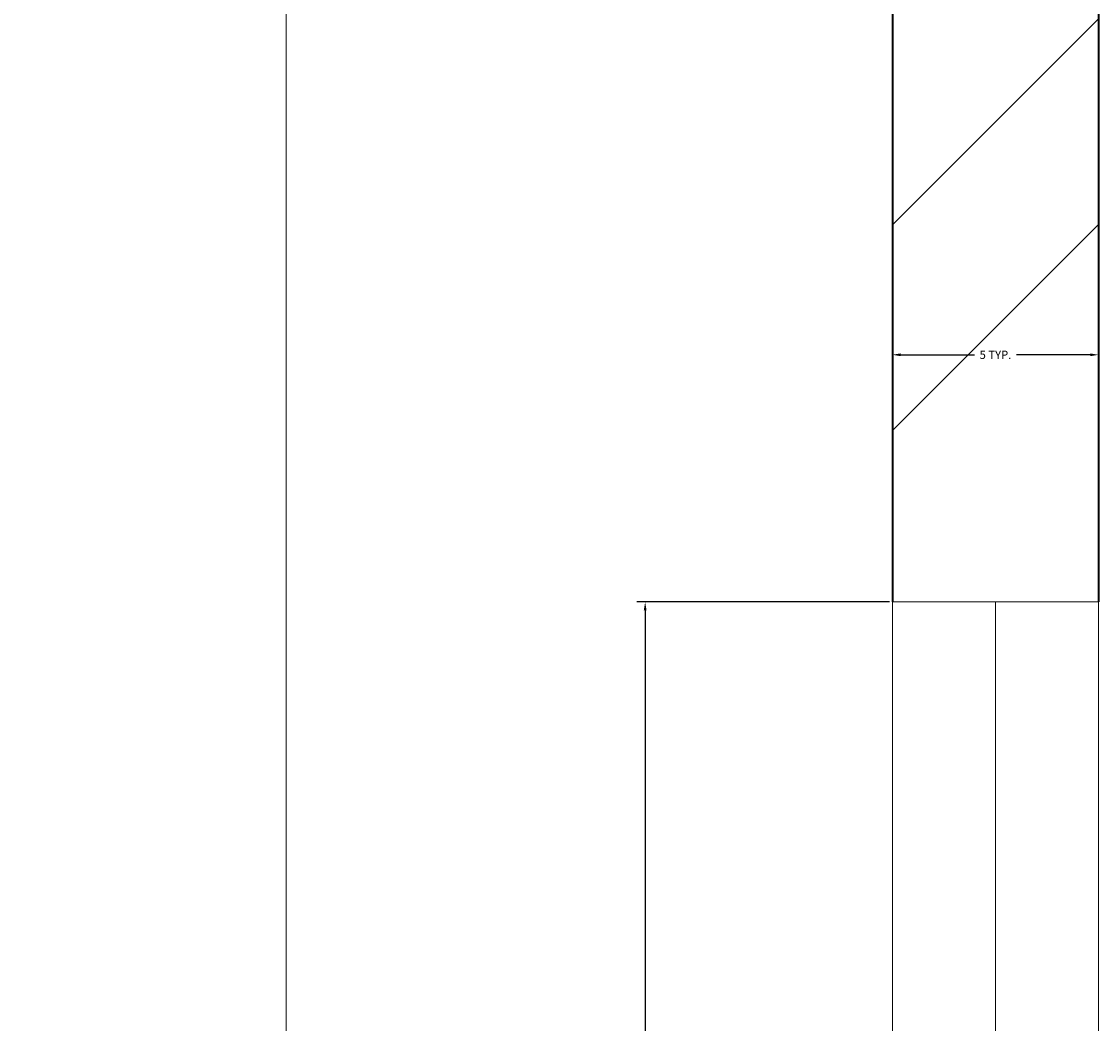
# Model space of a CAD drawing. Units: inches. Extents: x 1885 to 2748, y 783 to 2421.
# Tile 114 of 117: x 2595 to 2618, y 2071 to 2093. Entities that reach past the tile are written whole.
import ezdxf

# ---------------------------------------------------------------- set-up
doc = ezdxf.new("R2010")
doc.units = ezdxf.units.IN
for name, color, linetype, lineweight in [('A-ANNO-DIMS', 2, 'Continuous', 18), ('A-FLOR-CASE', 9, 'Continuous', 18), ('A-GLAZ', 181, 'Continuous', 18), ('A-WALL', 7, 'Continuous', 35)]:
    doc.layers.add(name, color=color, linetype=linetype, lineweight=lineweight)
doc.layers.add('A-WALL-PATT', color=85, linetype='Continuous', lineweight=13, true_color=0x58ba48)
doc.styles.get("Standard").update_dxf_attribs({"font": 'arial.ttf'})
doc.dimstyles.get("Standard").update_dxf_attribs({"dimtxt": 0.18, "dimasz": 0.18, "dimexe": 0.18, "dimexo": 0.0625, "dimgap": 0.09, "dimtad": 0, "dimtih": 1, "dimtoh": 1, "dimdec": 4, "dimzin": 0, "dimdsep": 46, "dimtxsty": 'Standard', "dimcen": 0.09, "dimadec": 0, "dimazin": 0, "dimtfac": 1, "dimtdec": 4, "dimtofl": 0, "dimtmove": 0, "dimatfit": 3, "dimfxl": 1, "dimtolj": 1, "dimtzin": 0, "dimarcsym": 0})

# ---------------------------------------------------------------- blocks, each defined once
blk = doc.blocks.new('WIN-36-ALT')
for p, q in [((0.004, 35.998), (4.504, 35.998)), ((0.004, 35.998), (0.004, -0.002)), ((4.504, 35.998), (2.254, 35.998)), ((2.254, 35.998), (2.254, -0.002)), ((4.504, -0.002), (4.504, 35.998)), ((4.504, -0.002), (0.004, -0.002)), ((2.254, -0.002), (4.504, -0.002))]:
    blk.add_line(p, q)
blk = doc.blocks.new('*D21')
at = {"layer": 'A-ANNO-DIMS', "color": 0, "lineweight": -2, "transparency": 16777216}
for p, q in [((2613.711, 2080.19), (2608.194, 2080.19)), ((2608.374, 2080.01), (2608.374, 2062.373)), ((2608.374, 2044.37), (2608.374, 2062.007)), ((2613.711, 2044.19), (2608.194, 2044.19))]:
    blk.add_line(p, q, dxfattribs=at)
at = {"layer": 'A-ANNO-DIMS', "color": 0, "transparency": 16777216}
for points in [[(2608.344, 2080.01), (2608.404, 2080.01), (2608.374, 2080.19)], [(2608.344, 2044.37), (2608.404, 2044.37), (2608.374, 2044.19)]]:
    blk.add_solid(points, dxfattribs=at)
at = {"layer": 'Defpoints', "color": 0, "transparency": 16777216}
for p in [(2608.374, 2080.19), (2613.774, 2080.19), (2613.774, 2044.19)]:
    blk.add_point(p, dxfattribs=at)
at = {"layer": 'A-ANNO-DIMS', "color": 0, "transparency": 16777216, "insert": (2608.374, 2062.19), "char_height": 0.18, "attachment_point": 5}
blk.add_mtext('\\A1;ALT. WINDOW 36 TYP.', dxfattribs=at)
blk = doc.blocks.new('*D22')
at = {"layer": 'A-ANNO-DIMS', "color": 0, "lineweight": -2, "transparency": 16777216}
for p, q in [((2613.774, 2080.252), (2613.774, 2085.77)), ((2618.274, 2080.252), (2618.274, 2085.77)), ((2613.954, 2085.59), (2615.565, 2085.59)), ((2618.094, 2085.59), (2616.482, 2085.59))]:
    blk.add_line(p, q, dxfattribs=at)
at = {"layer": 'A-ANNO-DIMS', "color": 0, "transparency": 16777216}
for points in [[(2613.954, 2085.62), (2613.954, 2085.56), (2613.774, 2085.59)], [(2618.094, 2085.62), (2618.094, 2085.56), (2618.274, 2085.59)]]:
    blk.add_solid(points, dxfattribs=at)
at = {"layer": 'Defpoints', "color": 0, "transparency": 16777216}
for p in [(2618.274, 2085.59), (2613.774, 2080.19), (2618.274, 2080.19)]:
    blk.add_point(p, dxfattribs=at)
at = {"layer": 'A-ANNO-DIMS', "color": 0, "transparency": 16777216, "insert": (2616.024, 2085.59), "char_height": 0.18, "attachment_point": 5}
blk.add_mtext('\\A1;5 TYP.', dxfattribs=at)

msp = doc.modelspace()

# ---------------------------------------------------------------- hatches: boundary and pattern name
at = {"layer": 'A-WALL-PATT'}
h = msp.add_hatch(dxfattribs=at)
h.set_pattern_fill('ANSI32', color=256)
h.paths.add_polyline_path([(2007.772, 2318.006), (1980.774, 2318.006), (1980.774, 2281.215), (1985.274, 2281.215), (1985.274, 2313.506), (2007.772, 2313.506), (2007.772, 2315.756)])
h.paths.add_polyline_path([(2094.324, 2318.006), (2067.772, 2318.006), (2067.772, 2313.506), (2094.324, 2313.506), (2094.324, 2315.756)])
h.paths.add_polyline_path([(2131.367, 2315.756), (2131.367, 2318.006), (2131.189, 2318.006), (2112.609, 2318.006), (2112.609, 2313.506), (2117.274, 2313.506), (2117.274, 2255.201), (2121.774, 2255.201), (2121.774, 2313.506), (2131.367, 2313.506)])
h.paths.add_polyline_path([(2190.512, 2318.006), (2155.367, 2318.006), (2155.367, 2313.506), (2169.774, 2313.506), (2169.774, 2229.506), (2121.774, 2229.506), (2121.774, 2233.451), (2119.524, 2233.451), (2117.274, 2233.451), (2117.274, 2201.101), (2121.774, 2201.101), (2121.774, 2225.006), (2169.774, 2225.006), (2169.774, 2165.006), (2306.274, 2165.006), (2306.274, 2066.006), (2310.774, 2066.006), (2344.274, 2066.006), (2486.274, 2066.006), (2486.274, 1886.006), (2483.02, 1886.006), (2483.02, 1881.506), (2486.274, 1881.506), (2486.274, 1880.678), (2490.774, 1880.678), (2490.774, 2070.506), (2344.274, 2070.506), (2310.774, 2070.506), (2310.774, 2165.006), (2310.774, 2173.636), (2308.524, 2173.636), (2306.274, 2173.636), (2306.274, 2169.506), (2174.274, 2169.506), (2174.274, 2313.506), (2190.512, 2313.506), (2190.512, 2315.756)])
h.paths.add_polyline_path([(1985.274, 2221.215), (1980.774, 2221.215), (1980.774, 2165.006), (1992.774, 2165.006), (1992.774, 2141.927), (1997.274, 2141.927), (1997.274, 2165.006), (2117.274, 2165.006), (2117.274, 2163.126), (2121.774, 2163.126), (2121.774, 2172.734), (2119.524, 2172.734), (2117.274, 2172.734), (2117.274, 2169.506), (1985.274, 2169.506)])
h.paths.add_polyline_path([(1997.274, 2105.927), (1992.774, 2105.927), (1992.774, 2070.506), (2016.774, 2070.506), (2016.774, 2059.123), (2019.024, 2059.123), (2021.274, 2059.123), (2021.274, 2070.506), (2117.274, 2070.506), (2117.274, 2022.506), (2114.423, 2022.506), (2114.423, 2018.006), (2123.627, 2018.006), (2123.627, 2020.256), (2123.627, 2022.506), (2121.774, 2022.506), (2121.774, 2142.587), (2119.524, 2142.587), (2117.274, 2142.587), (2117.274, 2075.006), (1997.274, 2075.006)])
h.paths.add_polyline_path([(2092.029, 2020.256), (2092.029, 2022.506), (2021.274, 2022.506), (2021.274, 2035.123), (2016.774, 2035.123), (2016.774, 2018.006), (2016.774, 1978.784), (2021.274, 1978.784), (2021.274, 2018.006), (2092.029, 2018.006)])
h.paths.add_polyline_path([(2260.938, 2022.506), (2153.105, 2022.506), (2153.105, 2020.256), (2153.105, 2018.006), (2155.274, 2018.006), (2155.274, 1886.006), (2107.629, 1886.006), (2107.629, 1881.506), (2182.911, 1881.506), (2182.911, 1883.756), (2182.911, 1886.006), (2159.774, 1886.006), (2159.774, 2018.006), (2260.938, 2018.006), (2260.938, 2020.256)])
h.paths.add_polyline_path([(2047.629, 1883.756), (2047.629, 1886.006), (2021.274, 1886.006), (2021.274, 1918.784), (2019.024, 1918.784), (2016.774, 1918.784), (2016.774, 1881.506), (2047.629, 1881.506)])
h.paths.add_polyline_path([(2306.361, 1883.756), (2306.361, 1886.006), (2296.274, 1886.006), (2296.274, 1982.006), (2316.535, 1982.006), (2316.535, 1984.256), (2316.535, 1986.506), (2296.274, 1986.506), (2296.274, 2022.506), (2289.276, 2022.506), (2289.276, 2018.006), (2291.774, 2018.006), (2291.774, 1886.006), (2242.911, 1886.006), (2242.911, 1881.506), (2306.361, 1881.506)], flags=17)
h.paths.add_polyline_path([(1985.274, 1843.006), (2021.6, 1843.006), (2021.534, 1845.441), (2021.477, 1847.506), (1980.774, 1847.506), (1980.774, 1809.446), (1985.274, 1809.446)])
h.paths.add_polyline_path([(2131.482, 1845.256), (2131.482, 1847.506), (2081.534, 1847.506), (2081.534, 1843.006), (2117.274, 1843.006), (2117.274, 1784.147), (2119.524, 1784.147), (2121.774, 1784.147), (2121.774, 1843.006), (2131.482, 1843.006)])
h.paths.add_polyline_path([(2203.886, 1847.506), (2155.482, 1847.506), (2155.482, 1843.006), (2169.774, 1843.006), (2169.774, 1759.006), (2121.774, 1759.006), (2121.774, 1761.457), (2117.274, 1761.457), (2117.274, 1730.429), (2121.774, 1730.429), (2121.774, 1754.506), (2177.421, 1754.506), (2177.421, 1756.756), (2177.421, 1759.006), (2174.274, 1759.006), (2174.274, 1843.006), (2203.886, 1843.006)])
h.paths.add_polyline_path([(2335.554, 1845.256), (2335.554, 1847.506), (2239.886, 1847.506), (2239.886, 1843.006), (2306.274, 1843.006), (2306.274, 1759.006), (2199.486, 1759.006), (2199.486, 1754.506), (2310.774, 1754.506), (2310.774, 1843.006), (2335.554, 1843.006)])
h.paths.add_polyline_path([(2348.774, 2022.506), (2344.274, 2022.506), (2344.274, 1986.506), (2341.681, 1986.506), (2341.681, 1982.006), (2344.274, 1982.006), (2344.274, 1886.006), (2330.361, 1886.006), (2330.361, 1881.506), (2361.627, 1881.506), (2361.627, 1883.756), (2361.627, 1886.006), (2348.774, 1886.006)], flags=17)
h.paths.add_polyline_path([(2283.251, 2315.756), (2283.251, 2318.006), (2238.512, 2318.006), (2238.512, 2313.506), (2283.251, 2313.506)], flags=17)
h.paths.add_polyline_path([(2363.274, 2348.006), (2388.677, 2348.006), (2388.677, 2350.256), (2388.677, 2352.506), (2358.774, 2352.506), (2358.774, 2348.006), (2358.774, 2318.006), (2344.481, 2318.006), (2344.481, 2313.506), (2358.774, 2313.506), (2358.774, 2229.506), (2310.774, 2229.506), (2310.774, 2231.952), (2306.274, 2231.952), (2306.274, 2205.611), (2310.774, 2205.611), (2310.774, 2225.006), (2358.774, 2225.006), (2358.774, 2211.506), (2452.329, 2211.506), (2452.329, 2213.756), (2452.329, 2216.006), (2363.274, 2216.006), (2363.274, 2318.006)])
h.paths.add_polyline_path([(2310.774, 2313.506), (2320.481, 2313.506), (2320.481, 2315.756), (2320.481, 2318.006), (2302.728, 2318.006), (2302.728, 2313.506), (2306.274, 2313.506), (2306.274, 2251.076), (2310.774, 2251.076)], flags=17)
h.paths.add_polyline_path([(2490.774, 2352.506), (2486.274, 2352.506), (2448.677, 2352.506), (2448.677, 2348.006), (2486.274, 2348.006), (2486.274, 2318.006), (2486.274, 2216.006), (2481.78, 2216.006), (2481.78, 2211.506), (2486.274, 2211.506), (2486.274, 2165.006), (2493.289, 2165.006), (2493.289, 2167.256), (2493.289, 2169.506), (2490.774, 2169.506), (2490.774, 2313.506), (2494.429, 2313.506), (2494.429, 2318.006), (2490.774, 2318.006)])
h.paths.add_polyline_path([(2534.653, 2318.006), (2515.691, 2318.006), (2515.691, 2313.506), (2534.653, 2313.506), (2534.653, 2315.756)])
h.paths.add_polyline_path([(2618.274, 2318.006), (2594.653, 2318.006), (2594.653, 2313.506), (2613.774, 2313.506), (2613.774, 2281.706), (2618.274, 2281.706)])
h.paths.add_polyline_path([(2618.274, 2221.706), (2613.774, 2221.706), (2613.774, 2169.506), (2554.019, 2169.506), (2554.019, 2165.006), (2613.774, 2165.006), (2613.774, 2152.878), (2618.274, 2152.878)])
h.paths.add_polyline_path([(2618.274, 2128.878), (2616.024, 2128.878), (2613.774, 2128.878), (2613.774, 2117.006), (2529.774, 2117.006), (2529.774, 2165.006), (2532.848, 2165.006), (2532.848, 2169.506), (2522.867, 2169.506), (2522.867, 2165.006), (2525.274, 2165.006), (2525.274, 2117.006), (2525.274, 2112.506), (2525.274, 2108.576), (2529.774, 2108.576), (2529.774, 2112.506), (2613.774, 2112.506), (2613.774, 2080.19), (2618.274, 2080.19)])
h.paths.add_polyline_path([(2618.274, 2044.19), (2616.024, 2044.19), (2613.774, 2044.19), (2613.774, 2015.506), (2529.774, 2015.506), (2529.774, 2088.582), (2527.524, 2088.582), (2525.274, 2088.582), (2525.274, 2011.006), (2613.774, 2011.006), (2613.774, 1956.755), (2618.274, 1956.755)])
h.paths.add_polyline_path([(2618.274, 1881.506), (2618.274, 1896.755), (2613.774, 1896.755), (2613.774, 1881.506), (2613.774, 1847.506), (2592.715, 1847.506), (2592.715, 1843.006), (2613.774, 1843.006), (2613.774, 1765.006), (2613.774, 1760.506), (2609.621, 1760.506), (2609.621, 1756.006), (2613.774, 1756.006), (2613.774, 1660.006), (2608.544, 1660.006), (2608.544, 1655.506), (2613.774, 1655.506), (2613.774, 1508.158), (2618.274, 1508.158)])
h.paths.add_polyline_path([(2565.774, 1843.006), (2568.997, 1843.006), (2568.997, 1847.506), (2490.774, 1847.506), (2490.774, 1849.7), (2488.524, 1849.7), (2486.274, 1849.7), (2486.274, 1847.506), (2477.274, 1847.506), (2477.274, 1838.506), (2477.274, 1821.493), (2486.274, 1821.493), (2486.274, 1838.506), (2561.274, 1838.506), (2561.274, 1765.006), (2486.274, 1765.006), (2486.274, 1786.157), (2477.274, 1786.157), (2477.274, 1765.006), (2477.274, 1756.006), (2486.274, 1756.006), (2565.774, 1756.006), (2585.621, 1756.006), (2585.621, 1758.256), (2585.621, 1760.506), (2565.774, 1760.506), (2565.774, 1765.006)])
h.paths.add_polyline_path([(2486.274, 1651.006), (2561.274, 1651.006), (2561.274, 1567.006), (2486.274, 1567.006), (2486.274, 1591.321), (2477.274, 1591.321), (2477.274, 1567.006), (2477.274, 1558.006), (2477.274, 1555.439), (2481.774, 1555.439), (2481.774, 1558.006), (2568.653, 1558.006), (2568.653, 1560.256), (2568.653, 1562.506), (2565.774, 1562.506), (2565.774, 1655.506), (2584.544, 1655.506), (2584.544, 1657.756), (2584.544, 1660.006), (2565.774, 1660.006), (2486.274, 1660.006), (2477.274, 1660.006), (2477.274, 1651.006), (2477.274, 1632.989), (2486.274, 1632.989)])
h.paths.add_polyline_path([(2449.967, 1883.756), (2449.967, 1886.006), (2421.627, 1886.006), (2421.627, 1881.506), (2449.967, 1881.506)], flags=17)
h.paths.add_polyline_path([(2447.274, 1847.506), (2395.554, 1847.506), (2395.554, 1843.006), (2442.774, 1843.006), (2442.774, 1809.27), (2447.274, 1809.27)])
h.paths.add_polyline_path([(1985.274, 1749.446), (1980.774, 1749.446), (1980.774, 1694.504), (1985.274, 1694.504), (1985.274, 1694.506), (1986.897, 1694.506), (1986.897, 1697.78), (1986.897, 1699.006), (1985.274, 1699.006)])
h.paths.add_polyline_path([(2152.774, 1699.006), (2121.774, 1699.006), (2121.774, 1703.668), (2119.524, 1703.668), (2117.274, 1703.668), (2117.274, 1699.006), (2009.219, 1699.006), (2009.219, 1694.506), (2148.274, 1694.506), (2148.274, 1692.631), (2152.774, 1692.631)])
h.paths.add_polyline_path([(2016.274, 1694.506), (2011.774, 1694.506), (2011.774, 1558.006), (2040.806, 1558.006), (2040.806, 1560.256), (2040.806, 1562.506), (2016.274, 1562.506)])
h.paths.add_polyline_path([(2152.774, 1663.017), (2150.524, 1663.017), (2148.274, 1663.017), (2148.274, 1562.506), (2100.806, 1562.506), (2100.806, 1558.006), (2165.119, 1558.006), (2165.119, 1560.256), (2165.119, 1562.506), (2152.774, 1562.506), (2152.774, 1610.506), (2224.774, 1610.506), (2224.774, 1607.99), (2229.274, 1607.99), (2229.274, 1615.006), (2152.774, 1615.006)])
h.paths.add_polyline_path([(2238.613, 1560.256), (2238.613, 1562.506), (2229.274, 1562.506), (2229.274, 1588.756), (2227.024, 1588.763), (2224.774, 1588.771), (2224.774, 1562.506), (2189.119, 1562.506), (2189.119, 1558.006), (2238.613, 1558.006)])
h.paths.add_polyline_path([(2336.024, 1560.256), (2336.024, 1562.506), (2310.774, 1562.506), (2310.774, 1656.347), (2308.524, 1656.347), (2306.274, 1656.347), (2306.274, 1562.506), (2286.613, 1562.506), (2286.613, 1558.006), (2336.024, 1558.006)])
h.paths.add_polyline_path([(2447.274, 1690.968), (2445.024, 1690.968), (2442.774, 1690.968), (2442.774, 1687.006), (2306.274, 1687.006), (2306.274, 1680.75), (2310.774, 1680.75), (2310.774, 1682.506), (2442.774, 1682.506), (2442.774, 1562.506), (2396.024, 1562.506), (2396.024, 1558.006), (2447.274, 1558.006)])
h.paths.add_polyline_path([(2447.274, 1749.27), (2445.024, 1749.27), (2442.774, 1749.27), (2442.774, 1717.232), (2447.274, 1717.232)])
h.paths.add_polyline_path([(2044.674, 1521.756), (2044.674, 1524.006), (2007.274, 1524.006), (2007.274, 1503.49), (2009.524, 1503.49), (2011.774, 1503.49), (2011.774, 1519.506), (2044.674, 1519.506)])
h.paths.add_polyline_path([(2177.969, 1521.756), (2177.969, 1524.006), (2104.674, 1524.006), (2104.674, 1519.506), (2145.774, 1519.506), (2145.774, 1387.506), (2143.37, 1387.506), (2143.37, 1383.006), (2251.585, 1383.006), (2251.585, 1385.256), (2251.585, 1387.506), (2150.274, 1387.506), (2150.274, 1519.506), (2177.969, 1519.506)])
h.paths.add_polyline_path([(2298.704, 1524.006), (2237.969, 1524.006), (2237.969, 1519.506), (2282.274, 1519.506), (2282.274, 1387.506), (2279.683, 1387.506), (2279.683, 1383.006), (2286.774, 1383.006), (2286.774, 1419.006), (2312.451, 1419.006), (2312.451, 1421.256), (2312.451, 1423.506), (2286.774, 1423.506), (2286.774, 1519.506), (2298.704, 1519.506), (2298.704, 1521.722)], flags=17)
h.paths.add_polyline_path([(2361.897, 1521.756), (2361.897, 1524.006), (2322.704, 1524.006), (2322.704, 1519.506), (2334.774, 1519.506), (2334.774, 1423.506), (2331.93, 1423.506), (2331.93, 1419.006), (2334.774, 1419.006), (2334.774, 1387.506), (2334.774, 1383.228), (2339.274, 1383.228), (2339.274, 1387.506), (2339.274, 1519.506), (2361.897, 1519.506)], flags=17)
h.paths.add_polyline_path([(2447.274, 1521.756), (2447.274, 1524.006), (2421.897, 1524.006), (2421.897, 1519.506), (2447.274, 1519.506)], flags=17)
h.paths.add_polyline_path([(2481.774, 1529.6), (2479.524, 1529.6), (2477.274, 1529.6), (2477.274, 1524.006), (2474.489, 1524.006), (2474.489, 1519.506), (2477.274, 1519.506), (2477.274, 1334.506), (2296.774, 1334.506), (2296.774, 1240.506), (2160.274, 1240.506), (2160.274, 1180.506), (2112.274, 1180.506), (2112.274, 1207.692), (2110.024, 1207.692), (2107.774, 1207.692), (2107.774, 1171.609), (2112.274, 1171.609), (2112.274, 1176.006), (2160.274, 1176.006), (2160.274, 1092.006), (2144.221, 1092.006), (2144.221, 1087.506), (2189.497, 1087.506), (2189.497, 1089.756), (2189.497, 1092.006), (2164.774, 1092.006), (2164.774, 1236.006), (2296.774, 1236.006), (2296.774, 1231.912), (2301.274, 1231.912), (2301.274, 1330.006), (2481.774, 1330.006), (2481.774, 1387.506)])
h.paths.add_polyline_path([(2618.274, 1448.158), (2613.774, 1448.158), (2613.774, 1382.506), (2529.774, 1382.506), (2525.274, 1382.506), (2525.274, 1307.062), (2529.774, 1307.062), (2529.774, 1378.006), (2613.774, 1378.006), (2613.774, 1354.988), (2618.274, 1354.988)])
h.paths.add_polyline_path([(2618.274, 1318.988), (2613.774, 1318.988), (2613.774, 1281.006), (2529.774, 1281.006), (2529.774, 1283.786), (2527.524, 1283.786), (2525.274, 1283.786), (2525.274, 1228.506), (2516.794, 1228.506), (2516.794, 1224.006), (2533.484, 1224.006), (2533.484, 1226.256), (2533.484, 1228.506), (2529.774, 1228.506), (2529.774, 1276.506), (2613.774, 1276.506), (2613.774, 1266.02), (2618.274, 1266.02)])
h.paths.add_polyline_path([(2618.274, 1134.964), (2613.774, 1134.964), (2613.774, 1092.006), (2594.545, 1092.006), (2594.545, 1087.506), (2618.274, 1087.506)])
h.paths.add_polyline_path([(2534.545, 1092.006), (2509.765, 1092.006), (2509.765, 1087.506), (2534.545, 1087.506), (2534.545, 1089.756)])
h.paths.add_polyline_path([(2481.274, 1224.006), (2484.117, 1224.006), (2484.117, 1226.256), (2484.117, 1228.506), (2476.774, 1228.506), (2476.774, 1198.506), (2471.61, 1198.506), (2471.61, 1194.006), (2476.774, 1194.006), (2476.774, 1062.006), (2436.894, 1062.006), (2436.894, 1057.506), (2476.774, 1057.506), (2481.274, 1057.506), (2481.274, 1062.006), (2481.274, 1087.506), (2485.354, 1087.506), (2485.354, 1089.756), (2485.354, 1092.006), (2481.274, 1092.006), (2481.274, 1117.506)])
h.paths.add_polyline_path([(2439.898, 1198.506), (2349.274, 1198.506), (2349.274, 1194.006), (2349.274, 1180.506), (2301.274, 1180.506), (2301.274, 1201.896), (2299.024, 1201.896), (2296.774, 1201.896), (2296.774, 1172.335), (2299.024, 1172.335), (2301.274, 1172.335), (2301.274, 1176.006), (2349.274, 1176.006), (2349.274, 1092.006), (2334.452, 1092.006), (2334.452, 1087.506), (2349.274, 1087.506), (2349.274, 1057.506), (2353.774, 1057.506), (2376.894, 1057.506), (2376.894, 1059.756), (2376.894, 1062.006), (2353.774, 1062.006), (2353.774, 1087.506), (2353.774, 1180.506), (2353.774, 1194.006), (2439.898, 1194.006), (2439.898, 1196.256)])
h.paths.add_polyline_path([(2270.596, 1089.756), (2270.596, 1092.006), (2249.497, 1092.006), (2249.497, 1087.506), (2270.596, 1087.506)], flags=17)
h.paths.add_polyline_path([(2310.452, 1092.006), (2301.274, 1092.006), (2301.274, 1153.292), (2296.774, 1153.292), (2296.774, 1092.006), (2293.786, 1092.006), (2293.786, 1087.506), (2310.452, 1087.506), (2310.452, 1089.756)], flags=17)
h.paths.add_polyline_path([(2112.274, 1150.328), (2110.024, 1150.328), (2107.774, 1150.328), (2107.774, 1092.006), (2104.465, 1092.006), (2104.465, 1087.506), (2120.221, 1087.506), (2120.221, 1089.756), (2120.221, 1092.006), (2112.274, 1092.006)])
h.paths.add_polyline_path([(2082.172, 1092.006), (2058.144, 1092.006), (2058.144, 1087.506), (2082.172, 1087.506), (2082.172, 1089.756)])
h.paths.add_polyline_path([(1975.774, 1145.638), (1971.274, 1145.638), (1971.274, 1087.506), (1980.774, 1087.506), (1998.144, 1087.506), (1998.144, 1089.756), (1998.144, 1092.006), (1985.274, 1092.006), (1975.774, 1092.006)])
h.paths.add_polyline_path([(2112.274, 1244.385), (2110.024, 1244.385), (2107.774, 1244.385), (2107.774, 1240.506), (1992.274, 1240.506), (1992.274, 1271.008), (1987.774, 1271.008), (1987.774, 1240.506), (1980.774, 1240.506), (1975.774, 1240.506), (1971.274, 1240.506), (1971.274, 1205.638), (1975.774, 1205.638), (1975.774, 1236.006), (2107.774, 1236.006), (2107.774, 1233.444), (2112.274, 1233.444), (2112.274, 1236.006)])
h.paths.add_polyline_path([(2112.274, 1383.006), (2114.783, 1383.006), (2114.783, 1385.256), (2114.783, 1387.506), (2102.476, 1387.506), (2102.476, 1383.006), (2107.774, 1383.006), (2107.774, 1335.006), (2011.774, 1335.006), (2011.774, 1349.939), (2007.274, 1349.939), (2007.274, 1335.006), (1987.774, 1335.006), (1987.774, 1330.506), (1987.774, 1307.008), (1992.274, 1307.008), (1992.274, 1330.506), (2007.274, 1330.506), (2107.774, 1330.506), (2107.774, 1264.711), (2112.274, 1264.711)])
h.paths.add_polyline_path([(2077.857, 1387.506), (2011.774, 1387.506), (2011.774, 1390.036), (2009.524, 1390.036), (2007.274, 1390.036), (2007.274, 1373.939), (2011.774, 1373.939), (2011.774, 1383.006), (2077.857, 1383.006)])
h.paths.add_polyline_path([(2011.774, 1443.49), (2007.274, 1443.49), (2007.274, 1410.248), (2011.774, 1410.248)])

# ---------------------------------------------------------------- linework, layer by layer
at = {"layer": 'A-FLOR-CASE'}
msp.add_line((2600.531, 2112.506), (2600.531, 2028.584), dxfattribs=at)
at = {"layer": 'A-WALL'}
for p, q in [((2618.274, 2128.878), (2618.274, 2080.19)), ((2613.774, 2112.506), (2613.774, 2080.19))]:
    msp.add_line(p, q, dxfattribs=at)

# ---------------------------------------------------------------- block references
at = {"layer": 'A-GLAZ'}
msp.add_blockref('WIN-36-ALT', (2613.77, 2044.192), dxfattribs=at)

# ---------------------------------------------------------------- dimensions: what is measured, and where the dimension line sits
at = {"layer": 'A-ANNO-DIMS'}
dim = msp.add_linear_dim(base=(2618.273597599, 2085.589908763), p1=(2613.773597599, 2080.189908763), p2=(2618.273597599, 2080.189908763), text='<> TYP.', dimstyle='Standard', override={"dimdec": 0, "dimlfac": 1, "dimrnd": 0, "dimzin": 0, "dimdsep": 46, "dimlunit": 2}, dxfattribs=at)
dim.commit()
dim.dimension.update_dxf_attribs({"geometry": '*D22', "text_midpoint": (2616.023597599, 2085.589908763)})
dim = msp.add_linear_dim(base=(2608.374, 2080.19), p1=(2613.774, 2044.19), p2=(2613.774, 2080.19), angle=90, text='ALT. WINDOW <> TYP.', dimstyle='Standard', override={"dimdec": 0, "dimlfac": 1, "dimrnd": 0, "dimzin": 0, "dimdsep": 46, "dimlunit": 2}, dxfattribs=at)
dim.commit()
dim.dimension.update_dxf_attribs({"geometry": '*D21', "text_midpoint": (2608.374, 2062.19)})

doc.saveas('drawing.dxf')
